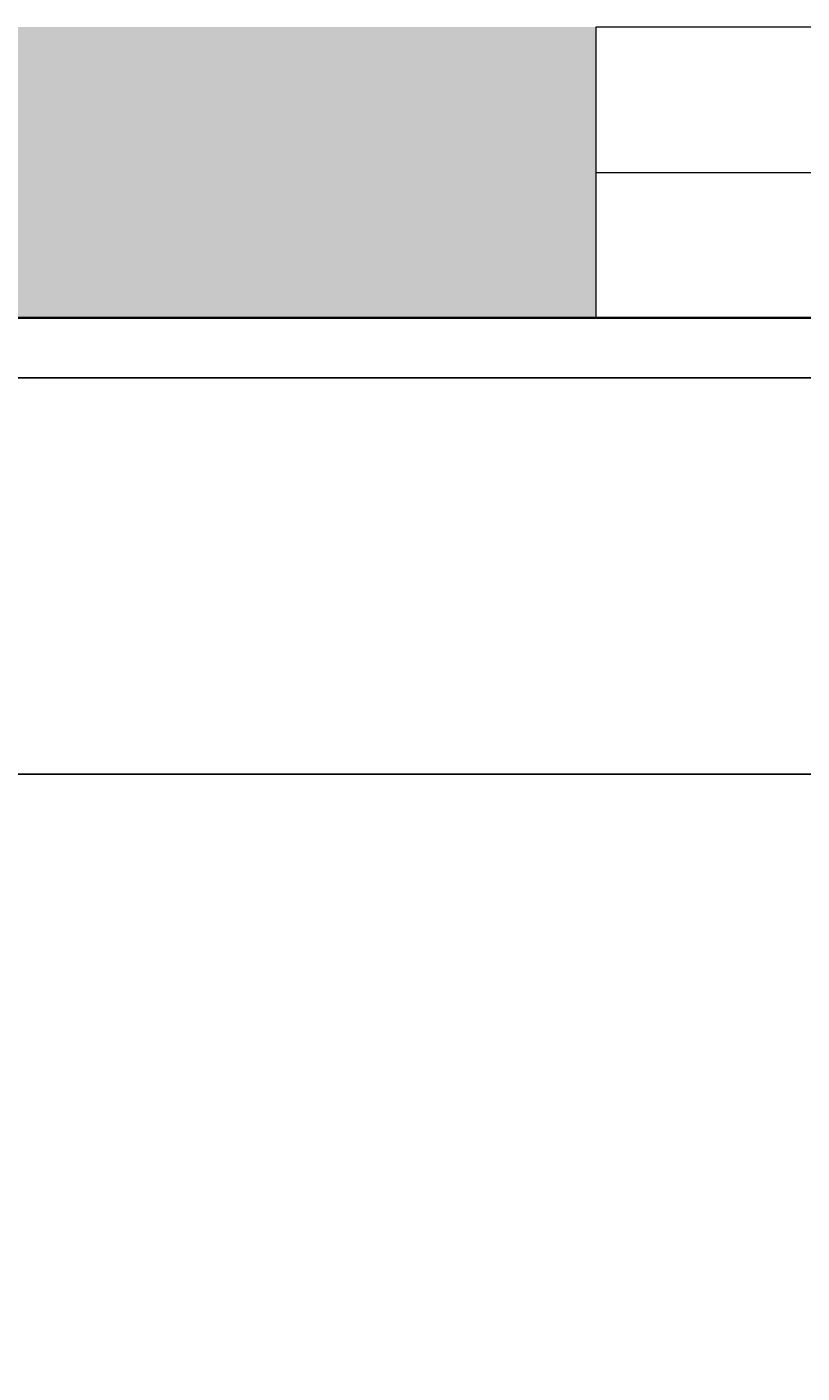
# Model space of a CAD drawing. Units: inches. Extents: x -5 to 482, y -460 to 66.
# Tile 24 of 31: x 48 to 72, y -29 to 13. Entities that reach past the tile are written whole.
import ezdxf

# ---------------------------------------------------------------- set-up
doc = ezdxf.new("R2010")
doc.units = ezdxf.units.IN
doc.header["$MEASUREMENT"] = 0
for name, color, linetype, lineweight in [('A-ANNO-DIMS', 2, 'Continuous', 18), ('A-GLAZ', 4, 'Continuous', 18), ('A-WALL', 7, 'Continuous', 35), ('A-WALL-PATT', 152, 'Continuous', 13)]:
    doc.layers.add(name, color=color, linetype=linetype, lineweight=lineweight)
doc.styles.get("Standard").update_dxf_attribs({"font": 'arial.ttf'})
doc.dimstyles.get("Standard").update_dxf_attribs({"dimtxt": 0.18, "dimasz": 0.18, "dimexe": 0.18, "dimexo": 0.0625, "dimgap": 0.09, "dimtad": 0, "dimtih": 1, "dimtoh": 1, "dimdec": 0, "dimzin": 0, "dimdsep": 46, "dimlunit": 3, "dimtxsty": 'Standard', "dimcen": 0.09, "dimadec": 0, "dimazin": 0, "dimtfac": 1, "dimtdec": 0, "dimtofl": 0, "dimtmove": 0, "dimatfit": 3, "dimfxl": 1, "dimtolj": 1, "dimtzin": 0, "dimarcsym": 0})

# ---------------------------------------------------------------- blocks, each defined once
blk = doc.blocks.new('WIN-GLAZ-60IN')
for p, q in [((0, 9), (60, 9)), ((0, 4.5), (60, 4.5)), ((60, 0), (0, 0))]:
    blk.add_line(p, q)
blk = doc.blocks.new('*D70')
at = {"layer": 'A-ANNO-DIMS', "color": 0, "lineweight": -2, "transparency": 16777216}
for p, q in [((83.652, 2.288), (-4.903, 2.288)), ((-4.723, 2.108), (-4.723, -3.659)), ((-4.723, -9.792), (-4.723, -4.025)), ((83.652, -9.972), (-4.903, -9.972))]:
    blk.add_line(p, q, dxfattribs=at)
at = {"layer": 'A-ANNO-DIMS', "color": 0, "transparency": 16777216}
for points in [[(-4.753, 2.108), (-4.693, 2.108), (-4.723, 2.288)], [(-4.753, -9.792), (-4.693, -9.792), (-4.723, -9.972)]]:
    blk.add_solid(points, dxfattribs=at)
at = {"layer": 'Defpoints', "color": 0, "transparency": 16777216}
for p in [(83.715, 2.288), (-4.723, -9.972), (83.715, -9.972)]:
    blk.add_point(p, dxfattribs=at)
at = {"layer": 'A-ANNO-DIMS', "color": 0, "transparency": 16777216, "insert": (-4.723, -3.842), "char_height": 0.18, "attachment_point": 5}
blk.add_mtext('\\A1;1\'-0 1/2"', dxfattribs=at)

msp = doc.modelspace()

# ---------------------------------------------------------------- hatches: boundary and pattern name
at = {"layer": 'A-WALL-PATT'}
h = msp.add_hatch(color=256, dxfattribs=at)
h.dxf.hatch_style = 1
h.paths.add_polyline_path([(149.377, -412.849), (144.377, -412.849), (144.377, -283.849), (144.377, -279.349), (133.877, -279.349), (133.877, -283.849), (139.877, -283.849), (139.877, -412.849), (133.51, -412.849), (133.51, -413.916), (102.652, -413.916), (102.652, -421.02), (133.51, -421.02), (133.51, -421.849), (149.377, -421.849)])
h.paths.add_polyline_path([(226.054, -412.849), (218.877, -412.849), (218.877, -350.849), (262.877, -350.849), (262.877, -386.849), (267.377, -386.849), (267.377, -283.849), (270.377, -283.849), (270.377, -279.349), (244.877, -279.349), (244.877, -283.849), (262.877, -283.849), (262.877, -346.349), (218.877, -346.349), (218.877, -283.849), (220.877, -283.849), (220.877, -279.349), (214.377, -279.349), (214.377, -283.849), (214.377, -412.849), (209.377, -412.849), (209.377, -421.849), (226.054, -421.849)])
h.paths.add_polyline_path([(315.815, -412.849), (250.054, -412.849), (250.054, -421.849), (315.815, -421.849)])
h.paths.add_polyline_path([(430.377, -378.349), (421.377, -378.349), (421.377, -412.849), (375.815, -412.849), (375.815, -421.849), (430.377, -421.849)])
h.paths.add_polyline_path([(78.691, -413.916), (47.68, -413.916), (47.68, -412.849), (41.877, -412.849), (41.877, -283.849), (109.877, -283.849), (109.877, -279.349), (41.877, -279.349), (41.877, -241.849), (32.877, -241.849), (32.877, -421.849), (47.68, -421.849), (47.68, -421.02), (78.691, -421.02)])
h.paths.add_polyline_path([(41.877, -144.349), (154.377, -144.349), (154.377, -137.849), (149.877, -137.849), (149.877, -139.849), (41.877, -139.849), (41.877, -97.849), (32.877, -97.849), (32.877, -181.849), (41.877, -181.849)])
h.paths.add_polyline_path([(430.377, -241.849), (421.377, -241.849), (421.377, -279.349), (309.377, -279.349), (309.377, -170.349), (304.877, -170.349), (304.877, -279.349), (294.377, -279.349), (294.377, -283.849), (421.377, -283.849), (421.377, -318.349), (430.377, -318.349)])
h.paths.add_polyline_path([(430.377, -119.849), (421.377, -119.849), (421.377, -139.849), (419.377, -139.849), (419.377, -144.349), (421.377, -144.349), (421.377, -181.849), (430.377, -181.849)])
h.paths.add_polyline_path([(395.377, -139.849), (377.377, -139.849), (377.377, -75.849), (421.377, -75.849), (421.377, -95.849), (430.377, -95.849), (430.377, -45.599), (421.377, -45.599), (421.377, -71.349), (377.377, -71.349), (377.377, -22.849), (372.877, -22.849), (372.877, -139.849), (242.877, -139.849), (242.877, -137.849), (238.377, -137.849), (238.377, -144.349), (304.877, -144.349), (304.877, -146.349), (309.377, -146.349), (309.377, -144.349), (395.377, -144.349)])
h.paths.add_polyline_path([(65.877, 13.151), (32.877, 13.151), (32.877, -37.849), (41.877, -37.849), (41.877, 4.151), (65.877, 4.151)])
h.paths.add_polyline_path([(166.377, 13.151), (125.877, 13.151), (125.877, 4.151), (149.877, 4.151), (149.877, -113.849), (154.377, -113.849), (154.377, 4.151), (166.377, 4.151)])
h.paths.add_polyline_path([(277.877, 13.151), (226.377, 13.151), (226.377, 4.151), (238.377, 4.151), (238.377, -113.849), (242.877, -113.849), (242.877, 4.151), (277.877, 4.151)])
h.paths.add_polyline_path([(430.377, 13.151), (337.877, 13.151), (337.877, 4.151), (372.877, 4.151), (372.877, 1.151), (377.377, 1.151), (377.377, 4.151), (421.377, 4.151), (421.377, -21.599), (430.377, -21.599)])

# ---------------------------------------------------------------- linework, layer by layer
at = {"layer": 'A-GLAZ'}
msp.add_line((65.877, 4.151), (65.877, 13.151), dxfattribs=at)
at = {"layer": 'A-WALL'}
msp.add_line((41.877, 4.151), (149.877, 4.151), dxfattribs=at)

# ---------------------------------------------------------------- block references
at = {"layer": 'A-GLAZ'}
msp.add_blockref('WIN-GLAZ-60IN', (65.877, 4.151), dxfattribs=at)

# ---------------------------------------------------------------- dimensions: what is measured, and where the dimension line sits
at = {"layer": 'A-ANNO-DIMS'}
dim = msp.add_linear_dim(base=(-4.723, -9.972), p1=(83.715, 2.288), p2=(83.715, -9.972), angle=90, dimstyle='Standard', override={"dimdec": 1, "dimlfac": 1, "dimrnd": 0, "dimzin": 1, "dimdsep": 46, "dimlunit": 4, "dimfrac": 2}, dxfattribs=at)
dim.commit()
dim.dimension.update_dxf_attribs({"geometry": '*D70', "text_midpoint": (-4.723, -3.842)})

doc.saveas('drawing.dxf')
